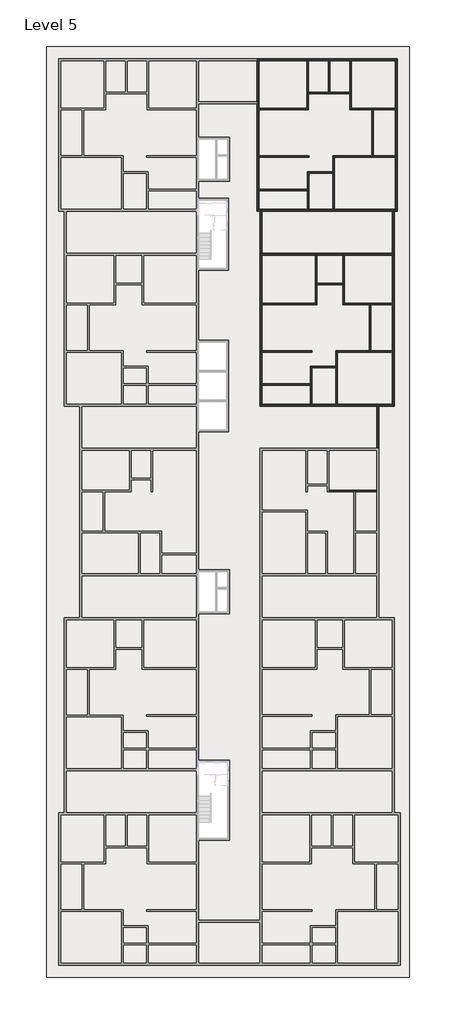
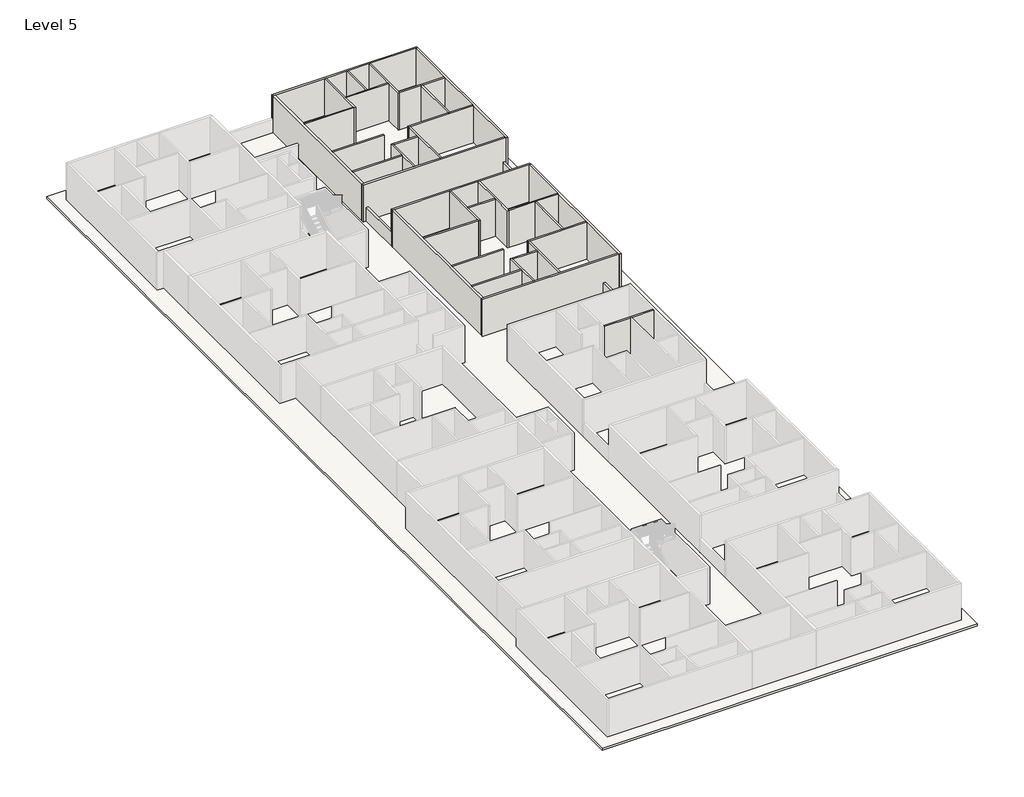
# One storey, part 4 of 8: 37 walls, 1 roof, 1 slab.
"""IFC4 building model written with IfcOpenShell, lengths in millimetres."""

from ifc_helpers import new_model, si_unit, frame, origin, place, context, project, spatial, polyline, outline, extrude, faceted_brep, element, save

model = new_model("IFC4")

# Units and contexts
model_context = context("Model", 3, world=origin())
ifc_project = project(units=[si_unit("LENGTHUNIT", "METRE", prefix="MILLI")], contexts=[model_context])

# Site, building, storey
site = spatial("IfcSite", under=ifc_project)
building = spatial("IfcBuilding", under=site)
storey = spatial("IfcBuildingStorey", under=building, Name="Level 5", Elevation=37426.6172466)

# Roof
placement = place(None, origin())
element("IfcRoof", 1, ObjectType="SLAB", at=placement, inside=storey, context=model_context, shape_type="SweptSolid", body=[
    extrude(outline(polyline([(-15237.9415084, -35021.5344126), (-15237.9415084, 36097.9216096), (12498.9443719, 36097.9216096), (12498.9443719, -35021.5344126), (-15237.9415084, -35021.5344126)]), holes=[polyline([(-3617.4415084, 29152.4900967), (-3617.4415084, 25799.6900967), (-1255.2415084, 25799.6900967), (-1255.2415084, 29152.4900967), (-3617.4415084, 29152.4900967)]), polyline([(-3617.4415084, 24490.1216096), (-3617.4415084, 19003.7216096), (-1331.4415084, 19003.7216096), (-1331.4415084, 24490.1216096), (-3617.4415084, 24490.1216096)]), polyline([(-3617.4415084, 13669.6303368), (-3617.4415084, 6659.2303368), (-1331.4415084, 6659.2303368), (-1331.4415084, 13669.6303368), (-3617.4415084, 13669.6303368)]), polyline([(-3617.4415084, -3882.2751812), (-3617.4415084, -7235.0751812), (-1255.2415084, -7235.0751812), (-1255.2415084, -3882.2751812), (-3617.4415084, -3882.2751812)]), polyline([(-3617.4415084, -18429.9851539), (-3617.4415084, -24525.9851539), (-1229.8415084, -24525.9851539), (-1229.8415084, -18429.9851539), (-3617.4415084, -18429.9851539)])]), frame((0.0, 0.0, 37426.6172466), z_axis=(0.0, 0.0, 1.0), x_axis=(1.0, 0.0, 0.0)), (0.0, 0.0, 1.0), 152.4),
])

# Slab
element("IfcSlab", 2, ObjectType="FLOOR", at=placement, inside=storey, context=model_context, shape_type="SweptSolid", body=[
    extrude(outline(polyline([(-14323.5415084, 35183.5216096), (11584.5443719, 35183.5216096), (11584.5443719, 23499.5216096), (11360.9214687, 23499.5216096), (11360.9214687, 8615.1216096), (10173.4714687, 8615.1216096), (10173.4714687, -7538.7344126), (11360.9214687, -7538.7344126), (11360.9214687, -22423.1344126), (11813.0584916, -22423.1344126), (11813.0584916, -34107.1344126), (11584.5443719, -34107.1344126), (-14323.5415084, -34107.1344126), (-14323.5415084, 35183.5216096)]), holes=[polyline([(-3617.4415084, 29152.4900967), (-3617.4415084, 25799.6900967), (-1255.2415084, 25799.6900967), (-1255.2415084, 29152.4900967), (-3617.4415084, 29152.4900967)]), polyline([(-3617.4415084, 24490.1216096), (-3617.4415084, 19003.7216096), (-1331.4415084, 19003.7216096), (-1331.4415084, 24490.1216096), (-3617.4415084, 24490.1216096)]), polyline([(-3617.4415084, 13669.6303368), (-3617.4415084, 6659.2303368), (-1331.4415084, 6659.2303368), (-1331.4415084, 13669.6303368), (-3617.4415084, 13669.6303368)]), polyline([(-3617.4415084, -3882.2751812), (-3617.4415084, -7235.0751812), (-1255.2415084, -7235.0751812), (-1255.2415084, -3882.2751812), (-3617.4415084, -3882.2751812)]), polyline([(-3617.4415084, -18429.9851539), (-3617.4415084, -24525.9851539), (-1229.8415084, -24525.9851539), (-1229.8415084, -18429.9851539), (-3617.4415084, -18429.9851539)])]), frame((0.0, 0.0, 36817.0172466), z_axis=(0.0, 0.0, 1.0), x_axis=(1.0, 0.0, 0.0)), (0.0, 0.0, 1.0), 609.6),
])

# Walls
element("IfcWall", 3, ObjectType="4.5\"", at=placement, inside=storey, context=model_context, shape_type="Brep", body=[
    faceted_brep([(6363.4714687, 2100.0216096, 37426.6172466), (8282.4584916, 2100.0216096, 37426.6172466), (8396.7584916, 2100.0216096, 37426.6172466), (10021.0714687, 2100.0216096, 37426.6172466), (10021.0714687, 2100.0216096, 40474.6172466), (8396.7584916, 2100.0216096, 40474.6172466), (8282.4584916, 2100.0216096, 40474.6172466), (6363.4714687, 2100.0216096, 40474.6172466), (6363.4714687, 2214.3216096, 37426.6172466), (6363.4714687, 2214.3216096, 40474.6172466), (10021.0714687, 2214.3216096, 40474.6172466), (10021.0714687, 2214.3216096, 37426.6172466)], [[[0, 1, 2, 3, 4, 5, 6, 7]], [[8, 9, 10, 11]], [[3, 2, 1, 0, 8, 11]], [[0, 7, 9, 8]], [[4, 3, 11, 10]], [[7, 6, 5, 4, 10, 9]]]),
])
element("IfcWall", 4, ObjectType="4.5\"", at=placement, inside=storey, context=model_context, shape_type="Brep", body=[
    faceted_brep([(5315.7214687, 20146.7216096, 37426.6172466), (5315.7214687, 16489.1216096, 37426.6172466), (5315.7214687, 16374.8216096, 37426.6172466), (5315.7214687, 16374.8216096, 40474.6172466), (5315.7214687, 16489.1216096, 40474.6172466), (5315.7214687, 20146.7216096, 40474.6172466), (5430.0214687, 20146.7216096, 37426.6172466), (5430.0214687, 20146.7216096, 40474.6172466), (5430.0214687, 18013.1216096, 40474.6172466), (5430.0214687, 17898.8216096, 40474.6172466), (5430.0214687, 16374.8216096, 40474.6172466), (5430.0214687, 16374.8216096, 37426.6172466), (5430.0214687, 17898.8216096, 37426.6172466), (5430.0214687, 18013.1216096, 37426.6172466)], [[[0, 1, 2, 3, 4, 5]], [[6, 7, 8, 9, 10, 11, 12, 13]], [[2, 1, 0, 6, 13, 12, 11]], [[0, 5, 7, 6]], [[3, 2, 11, 10]], [[5, 4, 3, 10, 9, 8, 7]]]),
])
element("IfcWall", 5, ObjectType="4.5\"", at=placement, inside=storey, context=model_context, shape_type="SweptSolid", body=[
    extrude(outline(polyline([(1259.3584916, 16489.1216096), (5315.7214687, 16489.1216096), (5315.7214687, 16374.8216096), (1259.3584916, 16374.8216096), (1259.3584916, 16489.1216096)])), frame((0.0, 0.0, 37426.6172466), z_axis=(0.0, 0.0, 1.0), x_axis=(1.0, 0.0, 0.0)), (0.0, 0.0, 1.0), 3048.0),
])
element("IfcWall", 6, ObjectType="4.5\"", at=placement, inside=storey, context=model_context, shape_type="SweptSolid", body=[
    extrude(outline(polyline([(7436.6214687, 17898.8216096), (5430.0214687, 17898.8216096), (5430.0214687, 18013.1216096), (7436.6214687, 18013.1216096), (7436.6214687, 17898.8216096)])), frame((0.0, 0.0, 37426.6172466), z_axis=(0.0, 0.0, 1.0), x_axis=(1.0, 0.0, 0.0)), (0.0, 0.0, 1.0), 3048.0),
])
element("IfcWall", 7, ObjectType="4.5\"", at=placement, inside=storey, context=model_context, shape_type="Brep", body=[
    faceted_brep([(7436.6214687, 20146.7216096, 37426.6172466), (7436.6214687, 18013.1216096, 37426.6172466), (7436.6214687, 17898.8216096, 37426.6172466), (7436.6214687, 16374.8216096, 37426.6172466), (7436.6214687, 16374.8216096, 40474.6172466), (7436.6214687, 17898.8216096, 40474.6172466), (7436.6214687, 18013.1216096, 40474.6172466), (7436.6214687, 20146.7216096, 40474.6172466), (7550.9214687, 20146.7216096, 37426.6172466), (7550.9214687, 20146.7216096, 40474.6172466), (7550.9214687, 16489.1216096, 40474.6172466), (7550.9214687, 16374.8216096, 40474.6172466), (7550.9214687, 16374.8216096, 37426.6172466), (7550.9214687, 16489.1216096, 37426.6172466)], [[[0, 1, 2, 3, 4, 5, 6, 7]], [[8, 9, 10, 11, 12, 13]], [[3, 2, 1, 0, 8, 13, 12]], [[0, 7, 9, 8]], [[4, 3, 12, 11]], [[7, 6, 5, 4, 11, 10, 9]]]),
])
element("IfcWall", 8, ObjectType="4.5\"", at=placement, inside=storey, context=model_context, shape_type="Brep", body=[
    faceted_brep([(7550.9214687, 16374.8216096, 37426.6172466), (9469.9084916, 16374.8216096, 37426.6172466), (9584.2084916, 16374.8216096, 37426.6172466), (11208.5214687, 16374.8216096, 37426.6172466), (11208.5214687, 16374.8216096, 40474.6172466), (9584.2084916, 16374.8216096, 40474.6172466), (9469.9084916, 16374.8216096, 40474.6172466), (7550.9214687, 16374.8216096, 40474.6172466), (7550.9214687, 16489.1216096, 37426.6172466), (7550.9214687, 16489.1216096, 40474.6172466), (11208.5214687, 16489.1216096, 40474.6172466), (11208.5214687, 16489.1216096, 37426.6172466)], [[[0, 1, 2, 3, 4, 5, 6, 7]], [[8, 9, 10, 11]], [[3, 2, 1, 0, 8, 11]], [[0, 7, 9, 8]], [[4, 3, 11, 10]], [[7, 6, 5, 4, 10, 9]]]),
])
element("IfcWall", 9, ObjectType="4.5\"", at=placement, inside=storey, context=model_context, shape_type="SweptSolid", body=[
    extrude(outline(polyline([(9469.9084916, 12869.6216096), (9469.9084916, 16374.8216096), (9584.2084916, 16374.8216096), (9584.2084916, 12869.6216096), (9469.9084916, 12869.6216096)])), frame((0.0, 0.0, 37426.6172466), z_axis=(0.0, 0.0, 1.0), x_axis=(1.0, 0.0, 0.0)), (0.0, 0.0, 1.0), 3048.0),
])
element("IfcWall", 10, ObjectType="4.5\"", at=placement, inside=storey, context=model_context, shape_type="Brep", body=[
    faceted_brep([(11208.5214687, 12869.6216096, 37426.6172466), (9584.2084916, 12869.6216096, 37426.6172466), (9469.9084916, 12869.6216096, 37426.6172466), (6885.4584916, 12869.6216096, 37426.6172466), (6885.4584916, 12869.6216096, 40474.6172466), (9469.9084916, 12869.6216096, 40474.6172466), (9584.2084916, 12869.6216096, 40474.6172466), (11208.5214687, 12869.6216096, 40474.6172466), (11208.5214687, 12755.3216096, 37426.6172466), (11208.5214687, 12755.3216096, 40474.6172466), (6999.7584916, 12755.3216096, 40474.6172466), (6885.4584916, 12755.3216096, 40474.6172466), (6885.4584916, 12755.3216096, 37426.6172466), (6999.7584916, 12755.3216096, 37426.6172466)], [[[0, 1, 2, 3, 4, 5, 6, 7]], [[8, 9, 10, 11, 12, 13]], [[3, 2, 1, 0, 8, 13, 12]], [[0, 7, 9, 8]], [[4, 3, 12, 11]], [[7, 6, 5, 4, 11, 10, 9]]]),
])
element("IfcWall", 11, ObjectType="4.5\"", at=placement, inside=storey, context=model_context, shape_type="Brep", body=[
    faceted_brep([(6885.4584916, 12755.3216096, 37426.6172466), (6885.4584916, 11663.1216096, 37426.6172466), (6885.4584916, 11548.8216096, 37426.6172466), (6885.4584916, 8767.5216096, 37426.6172466), (6885.4584916, 8767.5216096, 40474.6172466), (6885.4584916, 11548.8216096, 40474.6172466), (6885.4584916, 11663.1216096, 40474.6172466), (6885.4584916, 12755.3216096, 40474.6172466), (6999.7584916, 12755.3216096, 37426.6172466), (6999.7584916, 12755.3216096, 40474.6172466), (6999.7584916, 8767.5216096, 40474.6172466), (6999.7584916, 8767.5216096, 37426.6172466)], [[[0, 1, 2, 3, 4, 5, 6, 7]], [[8, 9, 10, 11]], [[3, 2, 1, 0, 8, 11]], [[0, 7, 9, 8]], [[4, 3, 11, 10]], [[7, 6, 5, 4, 10, 9]]]),
])
element("IfcWall", 12, ObjectType="4.5\"", at=placement, inside=storey, context=model_context, shape_type="Brep", body=[
    faceted_brep([(5056.6584916, 8767.5216096, 37426.6172466), (5056.6584916, 11548.8216096, 37426.6172466), (5056.6584916, 11663.1216096, 37426.6172466), (5056.6584916, 11663.1216096, 40474.6172466), (5056.6584916, 11548.8216096, 40474.6172466), (5056.6584916, 8767.5216096, 40474.6172466), (4942.3584916, 8767.5216096, 37426.6172466), (4942.3584916, 8767.5216096, 40474.6172466), (4942.3584916, 10215.3216096, 40474.6172466), (4942.3584916, 10329.6216096, 40474.6172466), (4942.3584916, 11663.1216096, 40474.6172466), (4942.3584916, 11663.1216096, 37426.6172466), (4942.3584916, 10329.6216096, 37426.6172466), (4942.3584916, 10215.3216096, 37426.6172466)], [[[0, 1, 2, 3, 4, 5]], [[6, 7, 8, 9, 10, 11, 12, 13]], [[2, 1, 0, 6, 13, 12, 11]], [[0, 5, 7, 6]], [[3, 2, 11, 10]], [[5, 4, 3, 10, 9, 8, 7]]]),
])
element("IfcWall", 13, ObjectType="4.5\"", at=placement, inside=storey, context=model_context, shape_type="SweptSolid", body=[
    extrude(outline(polyline([(6885.4584916, 11548.8216096), (5056.6584916, 11548.8216096), (5056.6584916, 11663.1216096), (6885.4584916, 11663.1216096), (6885.4584916, 11548.8216096)])), frame((0.0, 0.0, 37426.6172466), z_axis=(0.0, 0.0, 1.0), x_axis=(1.0, 0.0, 0.0)), (0.0, 0.0, 1.0), 3048.0),
])
element("IfcWall", 14, ObjectType="4.5\"", at=placement, inside=storey, context=model_context, shape_type="SweptSolid", body=[
    extrude(outline(polyline([(4942.3584916, 10215.3216096), (1259.3584916, 10215.3216096), (1259.3584916, 10329.6216096), (4942.3584916, 10329.6216096), (4942.3584916, 10215.3216096)])), frame((0.0, 0.0, 37426.6172466), z_axis=(0.0, 0.0, 1.0), x_axis=(1.0, 0.0, 0.0)), (0.0, 0.0, 1.0), 3048.0),
])
element("IfcWall", 15, ObjectType="4.5\"", at=placement, inside=storey, context=model_context, shape_type="SweptSolid", body=[
    extrude(outline(polyline([(5056.6584916, 12755.3216096), (1259.3584916, 12755.3216096), (1259.3584916, 12869.6216096), (5056.6584916, 12869.6216096), (5056.6584916, 12755.3216096)])), frame((0.0, 0.0, 37426.6172466), z_axis=(0.0, 0.0, 1.0), x_axis=(1.0, 0.0, 0.0)), (0.0, 0.0, 1.0), 3048.0),
])
element("IfcWall", 16, ObjectType="4.5\"", at=placement, inside=storey, context=model_context, shape_type="Brep", body=[
    faceted_brep([(4688.4443719, 35031.1216096, 37426.6172466), (4688.4443719, 31373.5216096, 37426.6172466), (4688.4443719, 31259.2216096, 37426.6172466), (4688.4443719, 31259.2216096, 40474.6172466), (4688.4443719, 31373.5216096, 40474.6172466), (4688.4443719, 35031.1216096, 40474.6172466), (4802.7443719, 35031.1216096, 37426.6172466), (4802.7443719, 35031.1216096, 40474.6172466), (4802.7443719, 32592.7216096, 40474.6172466), (4802.7443719, 32478.4216096, 40474.6172466), (4802.7443719, 31259.2216096, 40474.6172466), (4802.7443719, 31259.2216096, 37426.6172466), (4802.7443719, 32478.4216096, 37426.6172466), (4802.7443719, 32592.7216096, 37426.6172466)], [[[0, 1, 2, 3, 4, 5]], [[6, 7, 8, 9, 10, 11, 12, 13]], [[2, 1, 0, 6, 13, 12, 11]], [[0, 5, 7, 6]], [[3, 2, 11, 10]], [[5, 4, 3, 10, 9, 8, 7]]]),
])
element("IfcWall", 17, ObjectType="4.5\"", at=placement, inside=storey, context=model_context, shape_type="SweptSolid", body=[
    extrude(outline(polyline([(1030.8443719, 31373.5216096), (4688.4443719, 31373.5216096), (4688.4443719, 31259.2216096), (1030.8443719, 31259.2216096), (1030.8443719, 31373.5216096)])), frame((0.0, 0.0, 37426.6172466), z_axis=(0.0, 0.0, 1.0), x_axis=(1.0, 0.0, 0.0)), (0.0, 0.0, 1.0), 3048.0),
])
element("IfcWall", 18, ObjectType="4.5\"", at=placement, inside=storey, context=model_context, shape_type="Brep", body=[
    faceted_brep([(4802.7443719, 32478.4216096, 37426.6172466), (7965.0443719, 32478.4216096, 37426.6172466), (7965.0443719, 32478.4216096, 40474.6172466), (4802.7443719, 32478.4216096, 40474.6172466), (4802.7443719, 32592.7216096, 37426.6172466), (4802.7443719, 32592.7216096, 40474.6172466), (6326.7443719, 32592.7216096, 40474.6172466), (6441.0443719, 32592.7216096, 40474.6172466), (7965.0443719, 32592.7216096, 40474.6172466), (7965.0443719, 32592.7216096, 37426.6172466), (6441.0443719, 32592.7216096, 37426.6172466), (6326.7443719, 32592.7216096, 37426.6172466)], [[[0, 1, 2, 3]], [[4, 5, 6, 7, 8, 9, 10, 11]], [[1, 0, 4, 11, 10, 9]], [[0, 3, 5, 4]], [[2, 1, 9, 8]], [[3, 2, 8, 7, 6, 5]]]),
])
element("IfcWall", 19, ObjectType="4.5\"", at=placement, inside=storey, context=model_context, shape_type="SweptSolid", body=[
    extrude(outline(polyline([(6326.7443719, 32592.7216096), (6326.7443719, 35031.1216096), (6441.0443719, 35031.1216096), (6441.0443719, 32592.7216096), (6326.7443719, 32592.7216096)])), frame((0.0, 0.0, 37426.6172466), z_axis=(0.0, 0.0, 1.0), x_axis=(1.0, 0.0, 0.0)), (0.0, 0.0, 1.0), 3048.0),
])
element("IfcWall", 20, ObjectType="4.5\"", at=placement, inside=storey, context=model_context, shape_type="Brep", body=[
    faceted_brep([(7965.0443719, 35031.1216096, 37426.6172466), (7965.0443719, 32592.7216096, 37426.6172466), (7965.0443719, 32478.4216096, 37426.6172466), (7965.0443719, 31259.2216096, 37426.6172466), (7965.0443719, 31259.2216096, 40474.6172466), (7965.0443719, 32478.4216096, 40474.6172466), (7965.0443719, 32592.7216096, 40474.6172466), (7965.0443719, 35031.1216096, 40474.6172466), (8079.3443719, 35031.1216096, 37426.6172466), (8079.3443719, 35031.1216096, 40474.6172466), (8079.3443719, 31373.5216096, 40474.6172466), (8079.3443719, 31259.2216096, 40474.6172466), (8079.3443719, 31259.2216096, 37426.6172466), (8079.3443719, 31373.5216096, 37426.6172466)], [[[0, 1, 2, 3, 4, 5, 6, 7]], [[8, 9, 10, 11, 12, 13]], [[3, 2, 1, 0, 8, 13, 12]], [[0, 7, 9, 8]], [[4, 3, 12, 11]], [[7, 6, 5, 4, 11, 10, 9]]]),
])
element("IfcWall", 21, ObjectType="4.5\"", at=placement, inside=storey, context=model_context, shape_type="Brep", body=[
    faceted_brep([(8079.3443719, 31259.2216096, 37426.6172466), (9641.4443719, 31259.2216096, 37426.6172466), (9755.7443719, 31259.2216096, 37426.6172466), (11432.1443719, 31259.2216096, 37426.6172466), (11432.1443719, 31259.2216096, 40474.6172466), (9755.7443719, 31259.2216096, 40474.6172466), (9641.4443719, 31259.2216096, 40474.6172466), (8079.3443719, 31259.2216096, 40474.6172466), (8079.3443719, 31373.5216096, 37426.6172466), (8079.3443719, 31373.5216096, 40474.6172466), (11432.1443719, 31373.5216096, 40474.6172466), (11432.1443719, 31373.5216096, 37426.6172466)], [[[0, 1, 2, 3, 4, 5, 6, 7]], [[8, 9, 10, 11]], [[3, 2, 1, 0, 8, 11]], [[0, 7, 9, 8]], [[4, 3, 11, 10]], [[7, 6, 5, 4, 10, 9]]]),
])
element("IfcWall", 22, ObjectType="4.5\"", at=placement, inside=storey, context=model_context, shape_type="SweptSolid", body=[
    extrude(outline(polyline([(9641.4443719, 27754.0216096), (9641.4443719, 31259.2216096), (9755.7443719, 31259.2216096), (9755.7443719, 27754.0216096), (9641.4443719, 27754.0216096)])), frame((0.0, 0.0, 37426.6172466), z_axis=(0.0, 0.0, 1.0), x_axis=(1.0, 0.0, 0.0)), (0.0, 0.0, 1.0), 3048.0),
])
element("IfcWall", 23, ObjectType="4.5\"", at=placement, inside=storey, context=model_context, shape_type="Brep", body=[
    faceted_brep([(11432.1443719, 27754.0216096, 37426.6172466), (9755.7443719, 27754.0216096, 37426.6172466), (9641.4443719, 27754.0216096, 37426.6172466), (6656.9443719, 27754.0216096, 37426.6172466), (6656.9443719, 27754.0216096, 40474.6172466), (9641.4443719, 27754.0216096, 40474.6172466), (9755.7443719, 27754.0216096, 40474.6172466), (11432.1443719, 27754.0216096, 40474.6172466), (11432.1443719, 27639.7216096, 37426.6172466), (11432.1443719, 27639.7216096, 40474.6172466), (6771.2443719, 27639.7216096, 40474.6172466), (6656.9443719, 27639.7216096, 40474.6172466), (6656.9443719, 27639.7216096, 37426.6172466), (6771.2443719, 27639.7216096, 37426.6172466)], [[[0, 1, 2, 3, 4, 5, 6, 7]], [[8, 9, 10, 11, 12, 13]], [[3, 2, 1, 0, 8, 13, 12]], [[0, 7, 9, 8]], [[4, 3, 12, 11]], [[7, 6, 5, 4, 11, 10, 9]]]),
])
element("IfcWall", 24, ObjectType="4.5\"", at=placement, inside=storey, context=model_context, shape_type="Brep", body=[
    faceted_brep([(6656.9443719, 27639.7216096, 37426.6172466), (6656.9443719, 26547.5216096, 37426.6172466), (6656.9443719, 26433.2216096, 37426.6172466), (6656.9443719, 23651.9216096, 37426.6172466), (6656.9443719, 23651.9216096, 40474.6172466), (6656.9443719, 26433.2216096, 40474.6172466), (6656.9443719, 26547.5216096, 40474.6172466), (6656.9443719, 27639.7216096, 40474.6172466), (6771.2443719, 27639.7216096, 37426.6172466), (6771.2443719, 27639.7216096, 40474.6172466), (6771.2443719, 23651.9216096, 40474.6172466), (6771.2443719, 23651.9216096, 37426.6172466)], [[[0, 1, 2, 3, 4, 5, 6, 7]], [[8, 9, 10, 11]], [[3, 2, 1, 0, 8, 11]], [[0, 7, 9, 8]], [[4, 3, 11, 10]], [[7, 6, 5, 4, 10, 9]]]),
])
element("IfcWall", 25, ObjectType="4.5\"", at=placement, inside=storey, context=model_context, shape_type="SweptSolid", body=[
    extrude(outline(polyline([(4713.8443719, 25099.7216096), (1030.8443719, 25099.7216096), (1030.8443719, 25214.0216096), (4713.8443719, 25214.0216096), (4713.8443719, 25099.7216096)])), frame((0.0, 0.0, 37426.6172466), z_axis=(0.0, 0.0, 1.0), x_axis=(1.0, 0.0, 0.0)), (0.0, 0.0, 1.0), 3048.0),
])
element("IfcWall", 26, ObjectType="4.5\"", at=placement, inside=storey, context=model_context, shape_type="Brep", body=[
    faceted_brep([(4828.1443719, 23651.9216096, 37426.6172466), (4828.1443719, 26433.2216096, 37426.6172466), (4828.1443719, 26547.5216096, 37426.6172466), (4828.1443719, 26547.5216096, 40474.6172466), (4828.1443719, 26433.2216096, 40474.6172466), (4828.1443719, 23651.9216096, 40474.6172466), (4713.8443719, 23651.9216096, 37426.6172466), (4713.8443719, 23651.9216096, 40474.6172466), (4713.8443719, 25099.7216096, 40474.6172466), (4713.8443719, 25214.0216096, 40474.6172466), (4713.8443719, 26547.5216096, 40474.6172466), (4713.8443719, 26547.5216096, 37426.6172466), (4713.8443719, 25214.0216096, 37426.6172466), (4713.8443719, 25099.7216096, 37426.6172466)], [[[0, 1, 2, 3, 4, 5]], [[6, 7, 8, 9, 10, 11, 12, 13]], [[2, 1, 0, 6, 13, 12, 11]], [[0, 5, 7, 6]], [[3, 2, 11, 10]], [[5, 4, 3, 10, 9, 8, 7]]]),
])
element("IfcWall", 27, ObjectType="4.5\"", at=placement, inside=storey, context=model_context, shape_type="SweptSolid", body=[
    extrude(outline(polyline([(6656.9443719, 26433.2216096), (4828.1443719, 26433.2216096), (4828.1443719, 26547.5216096), (6656.9443719, 26547.5216096), (6656.9443719, 26433.2216096)])), frame((0.0, 0.0, 37426.6172466), z_axis=(0.0, 0.0, 1.0), x_axis=(1.0, 0.0, 0.0)), (0.0, 0.0, 1.0), 3048.0),
])
element("IfcWall", 28, ObjectType="4.5\"", at=placement, inside=storey, context=model_context, shape_type="SweptSolid", body=[
    extrude(outline(polyline([(4828.1443719, 27639.7216096), (1030.8443719, 27639.7216096), (1030.8443719, 27754.0216096), (4828.1443719, 27754.0216096), (4828.1443719, 27639.7216096)])), frame((0.0, 0.0, 37426.6172466), z_axis=(0.0, 0.0, 1.0), x_axis=(1.0, 0.0, 0.0)), (0.0, 0.0, 1.0), 3048.0),
])
element("IfcWall", 29, ObjectType="6\"", at=placement, inside=storey, context=model_context, shape_type="Brep", body=[
    faceted_brep([(1106.9584916, 20146.7216096, 40474.6172466), (1106.9584916, 20146.7216096, 37426.6172466), (1259.3584916, 20146.7216096, 37426.6172466), (5315.7214687, 20146.7216096, 37426.6172466), (5430.0214687, 20146.7216096, 37426.6172466), (7436.6214687, 20146.7216096, 37426.6172466), (7550.9214687, 20146.7216096, 37426.6172466), (11208.5214687, 20146.7216096, 37426.6172466), (11360.9214687, 20146.7216096, 37426.6172466), (11360.9214687, 20146.7216096, 40474.6172466), (11208.5214687, 20146.7216096, 40474.6172466), (7550.9214687, 20146.7216096, 40474.6172466), (7436.6214687, 20146.7216096, 40474.6172466), (5430.0214687, 20146.7216096, 40474.6172466), (5315.7214687, 20146.7216096, 40474.6172466), (1259.3584916, 20146.7216096, 40474.6172466), (1106.9584916, 20299.1216096, 37426.6172466), (1106.9584916, 20299.1216096, 38645.8172466), (1106.9584916, 20299.1216096, 40474.6172466), (11360.9214687, 20299.1216096, 40474.6172466), (11360.9214687, 20299.1216096, 38645.8172466), (11360.9214687, 20299.1216096, 37426.6172466), (11208.5214687, 20299.1216096, 37426.6172466), (1259.3584916, 20299.1216096, 37426.6172466)], [[[0, 1, 2, 3, 4, 5, 6, 7, 8, 9, 10, 11, 12, 13, 14, 15]], [[16, 17, 18, 19, 20, 21, 22, 23]], [[8, 7, 6, 5, 4, 3, 2, 1, 16, 23, 22, 21]], [[0, 18, 17, 16, 1]], [[8, 21, 20, 19, 9]], [[0, 15, 14, 13, 12, 11, 10, 9, 19, 18]]]),
])
element("IfcWall", 30, ObjectType="6\"", at=placement, inside=storey, context=model_context, shape_type="Brep", body=[
    faceted_brep([(11208.5214687, 20146.7216096, 40474.6172466), (11208.5214687, 20146.7216096, 37426.6172466), (11208.5214687, 16489.1216096, 37426.6172466), (11208.5214687, 16374.8216096, 37426.6172466), (11208.5214687, 12869.6216096, 37426.6172466), (11208.5214687, 12755.3216096, 37426.6172466), (11208.5214687, 8767.5216096, 37426.6172466), (11208.5214687, 8615.1216096, 37426.6172466), (11208.5214687, 8615.1216096, 40474.6172466), (11208.5214687, 8767.5216096, 40474.6172466), (11208.5214687, 12755.3216096, 40474.6172466), (11208.5214687, 12869.6216096, 40474.6172466), (11208.5214687, 16374.8216096, 40474.6172466), (11208.5214687, 16489.1216096, 40474.6172466), (11360.9214687, 20146.7216096, 37426.6172466), (11360.9214687, 20146.7216096, 40474.6172466), (11360.9214687, 8615.1216096, 40474.6172466), (11360.9214687, 8615.1216096, 37426.6172466)], [[[0, 1, 2, 3, 4, 5, 6, 7, 8, 9, 10, 11, 12, 13]], [[14, 15, 16, 17]], [[7, 6, 5, 4, 3, 2, 1, 14, 17]], [[8, 7, 17, 16]], [[0, 15, 14, 1]], [[0, 13, 12, 11, 10, 9, 8, 16, 15]]]),
])
element("IfcWall", 31, ObjectType="6\"", at=placement, inside=storey, context=model_context, shape_type="Brep", body=[
    faceted_brep([(11208.5214687, 8767.5216096, 37426.6172466), (6999.7584916, 8767.5216096, 37426.6172466), (6885.4584916, 8767.5216096, 37426.6172466), (5056.6584916, 8767.5216096, 37426.6172466), (4942.3584916, 8767.5216096, 37426.6172466), (1259.3584916, 8767.5216096, 37426.6172466), (1106.9584916, 8767.5216096, 37426.6172466), (1106.9584916, 8767.5216096, 40474.6172466), (1259.3584916, 8767.5216096, 40474.6172466), (4942.3584916, 8767.5216096, 40474.6172466), (5056.6584916, 8767.5216096, 40474.6172466), (6885.4584916, 8767.5216096, 40474.6172466), (6999.7584916, 8767.5216096, 40474.6172466), (11208.5214687, 8767.5216096, 40474.6172466), (11208.5214687, 8615.1216096, 37426.6172466), (11208.5214687, 8615.1216096, 40474.6172466), (1106.9584916, 8615.1216096, 40474.6172466), (1106.9584916, 8615.1216096, 37426.6172466), (10021.0714687, 8615.1216096, 37426.6172466), (10173.4714687, 8615.1216096, 37426.6172466)], [[[0, 1, 2, 3, 4, 5, 6, 7, 8, 9, 10, 11, 12, 13]], [[14, 15, 16, 17, 18, 19]], [[6, 5, 4, 3, 2, 1, 0, 14, 19, 18, 17]], [[0, 13, 15, 14]], [[7, 6, 17, 16]], [[13, 12, 11, 10, 9, 8, 7, 16, 15]]]),
])
element("IfcWall", 32, ObjectType="6\"", at=placement, inside=storey, context=model_context, shape_type="Brep", body=[
    faceted_brep([(1259.3584916, 8767.5216096, 37426.6172466), (1259.3584916, 10215.3216096, 37426.6172466), (1259.3584916, 10329.6216096, 37426.6172466), (1259.3584916, 12755.3216096, 37426.6172466), (1259.3584916, 12869.6216096, 37426.6172466), (1259.3584916, 16374.8216096, 37426.6172466), (1259.3584916, 16489.1216096, 37426.6172466), (1259.3584916, 20146.7216096, 37426.6172466), (1259.3584916, 20146.7216096, 40474.6172466), (1259.3584916, 16489.1216096, 40474.6172466), (1259.3584916, 16374.8216096, 40474.6172466), (1259.3584916, 12869.6216096, 40474.6172466), (1259.3584916, 12755.3216096, 40474.6172466), (1259.3584916, 10329.6216096, 40474.6172466), (1259.3584916, 10215.3216096, 40474.6172466), (1259.3584916, 8767.5216096, 40474.6172466), (1106.9584916, 8767.5216096, 37426.6172466), (1106.9584916, 8767.5216096, 40474.6172466), (1106.9584916, 20146.7216096, 40474.6172466), (1106.9584916, 20146.7216096, 37426.6172466)], [[[0, 1, 2, 3, 4, 5, 6, 7, 8, 9, 10, 11, 12, 13, 14, 15]], [[16, 17, 18, 19]], [[7, 6, 5, 4, 3, 2, 1, 0, 16, 19]], [[0, 15, 17, 16]], [[7, 19, 18, 8]], [[15, 14, 13, 12, 11, 10, 9, 8, 18, 17]]]),
])
element("IfcWall", 33, ObjectType="6\"", at=placement, inside=storey, context=model_context, shape_type="Brep", body=[
    faceted_brep([(878.4443719, 35031.1216096, 40474.6172466), (878.4443719, 35031.1216096, 37426.6172466), (1030.8443719, 35031.1216096, 37426.6172466), (4688.4443719, 35031.1216096, 37426.6172466), (4802.7443719, 35031.1216096, 37426.6172466), (6326.7443719, 35031.1216096, 37426.6172466), (6441.0443719, 35031.1216096, 37426.6172466), (7965.0443719, 35031.1216096, 37426.6172466), (8079.3443719, 35031.1216096, 37426.6172466), (11432.1443719, 35031.1216096, 37426.6172466), (11584.5443719, 35031.1216096, 37426.6172466), (11584.5443719, 35031.1216096, 40474.6172466), (11432.1443719, 35031.1216096, 40474.6172466), (8079.3443719, 35031.1216096, 40474.6172466), (7965.0443719, 35031.1216096, 40474.6172466), (6441.0443719, 35031.1216096, 40474.6172466), (6326.7443719, 35031.1216096, 40474.6172466), (4802.7443719, 35031.1216096, 40474.6172466), (4688.4443719, 35031.1216096, 40474.6172466), (1030.8443719, 35031.1216096, 40474.6172466), (878.4443719, 35183.5216096, 37426.6172466), (878.4443719, 35183.5216096, 40474.6172466), (11584.5443719, 35183.5216096, 40474.6172466), (11584.5443719, 35183.5216096, 37426.6172466)], [[[0, 1, 2, 3, 4, 5, 6, 7, 8, 9, 10, 11, 12, 13, 14, 15, 16, 17, 18, 19]], [[20, 21, 22, 23]], [[10, 9, 8, 7, 6, 5, 4, 3, 2, 1, 20, 23]], [[11, 10, 23, 22]], [[0, 21, 20, 1]], [[0, 19, 18, 17, 16, 15, 14, 13, 12, 11, 22, 21]]]),
])
element("IfcWall", 34, ObjectType="6\"", at=placement, inside=storey, context=model_context, shape_type="Brep", body=[
    faceted_brep([(11432.1443719, 35031.1216096, 37426.6172466), (11432.1443719, 31373.5216096, 37426.6172466), (11432.1443719, 31259.2216096, 37426.6172466), (11432.1443719, 27754.0216096, 37426.6172466), (11432.1443719, 27639.7216096, 37426.6172466), (11432.1443719, 23651.9216096, 37426.6172466), (11432.1443719, 23499.5216096, 37426.6172466), (11432.1443719, 23499.5216096, 40474.6172466), (11432.1443719, 23651.9216096, 40474.6172466), (11432.1443719, 27639.7216096, 40474.6172466), (11432.1443719, 27754.0216096, 40474.6172466), (11432.1443719, 31259.2216096, 40474.6172466), (11432.1443719, 31373.5216096, 40474.6172466), (11432.1443719, 35031.1216096, 40474.6172466), (11584.5443719, 35031.1216096, 37426.6172466), (11584.5443719, 35031.1216096, 40474.6172466), (11584.5443719, 23499.5216096, 40474.6172466), (11584.5443719, 23499.5216096, 37426.6172466)], [[[0, 1, 2, 3, 4, 5, 6, 7, 8, 9, 10, 11, 12, 13]], [[14, 15, 16, 17]], [[6, 5, 4, 3, 2, 1, 0, 14, 17]], [[0, 13, 15, 14]], [[7, 6, 17, 16]], [[13, 12, 11, 10, 9, 8, 7, 16, 15]]]),
])
element("IfcWall", 35, ObjectType="6\"", at=placement, inside=storey, context=model_context, shape_type="Brep", body=[
    faceted_brep([(11432.1443719, 23651.9216096, 37426.6172466), (6771.2443719, 23651.9216096, 37426.6172466), (6656.9443719, 23651.9216096, 37426.6172466), (4828.1443719, 23651.9216096, 37426.6172466), (4713.8443719, 23651.9216096, 37426.6172466), (1030.8443719, 23651.9216096, 37426.6172466), (878.4443719, 23651.9216096, 37426.6172466), (878.4443719, 23651.9216096, 40474.6172466), (1030.8443719, 23651.9216096, 40474.6172466), (4713.8443719, 23651.9216096, 40474.6172466), (4828.1443719, 23651.9216096, 40474.6172466), (6656.9443719, 23651.9216096, 40474.6172466), (6771.2443719, 23651.9216096, 40474.6172466), (11432.1443719, 23651.9216096, 40474.6172466), (11432.1443719, 23499.5216096, 37426.6172466), (11432.1443719, 23499.5216096, 40474.6172466), (878.4443719, 23499.5216096, 40474.6172466), (878.4443719, 23499.5216096, 37426.6172466), (1106.9584916, 23499.5216096, 37426.6172466), (1259.3584916, 23499.5216096, 37426.6172466), (11208.5214687, 23499.5216096, 37426.6172466), (11360.9214687, 23499.5216096, 37426.6172466)], [[[0, 1, 2, 3, 4, 5, 6, 7, 8, 9, 10, 11, 12, 13]], [[14, 15, 16, 17, 18, 19, 20, 21]], [[6, 5, 4, 3, 2, 1, 0, 14, 21, 20, 19, 18, 17]], [[0, 13, 15, 14]], [[7, 6, 17, 16]], [[13, 12, 11, 10, 9, 8, 7, 16, 15]]]),
])
element("IfcWall", 36, ObjectType="6\"", at=placement, inside=storey, context=model_context, shape_type="Brep", body=[
    faceted_brep([(1030.8443719, 23651.9216096, 37426.6172466), (1030.8443719, 25099.7216096, 37426.6172466), (1030.8443719, 25214.0216096, 37426.6172466), (1030.8443719, 27639.7216096, 37426.6172466), (1030.8443719, 27754.0216096, 37426.6172466), (1030.8443719, 31259.2216096, 37426.6172466), (1030.8443719, 31373.5216096, 37426.6172466), (1030.8443719, 35031.1216096, 37426.6172466), (1030.8443719, 35031.1216096, 40474.6172466), (1030.8443719, 31373.5216096, 40474.6172466), (1030.8443719, 31259.2216096, 40474.6172466), (1030.8443719, 27754.0216096, 40474.6172466), (1030.8443719, 27639.7216096, 40474.6172466), (1030.8443719, 25214.0216096, 40474.6172466), (1030.8443719, 25099.7216096, 40474.6172466), (1030.8443719, 23651.9216096, 40474.6172466), (878.4443719, 23651.9216096, 37426.6172466), (878.4443719, 23651.9216096, 40474.6172466), (878.4443719, 35031.1216096, 40474.6172466), (878.4443719, 35031.1216096, 37426.6172466), (878.4443719, 31897.3197155, 37426.6172466), (878.4443719, 31744.9197155, 37426.6172466)], [[[0, 1, 2, 3, 4, 5, 6, 7, 8, 9, 10, 11, 12, 13, 14, 15]], [[16, 17, 18, 19, 20, 21]], [[7, 6, 5, 4, 3, 2, 1, 0, 16, 21, 20, 19]], [[0, 15, 17, 16]], [[7, 19, 18, 8]], [[15, 14, 13, 12, 11, 10, 9, 8, 18, 17]]]),
])
element("IfcWall", 37, ObjectType="6\" 2", at=placement, inside=storey, context=model_context, shape_type="SweptSolid", body=[
    extrude(outline(polyline([(1106.9584916, 20299.1216096), (1106.9584916, 23499.5216096), (1259.3584916, 23499.5216096), (1259.3584916, 20299.1216096), (1106.9584916, 20299.1216096)])), frame((0.0, 0.0, 37426.6172466), z_axis=(0.0, 0.0, 1.0), x_axis=(1.0, 0.0, 0.0)), (0.0, 0.0, 1.0), 1219.2),
])
element("IfcWall", 38, ObjectType="6\" 2", at=placement, inside=storey, context=model_context, shape_type="SweptSolid", body=[
    extrude(outline(polyline([(11208.5214687, 20299.1216096), (11208.5214687, 23499.5216096), (11360.9214687, 23499.5216096), (11360.9214687, 20299.1216096), (11208.5214687, 20299.1216096)])), frame((0.0, 0.0, 37426.6172466), z_axis=(0.0, 0.0, 1.0), x_axis=(1.0, 0.0, 0.0)), (0.0, 0.0, 1.0), 1219.2),
])
element("IfcWall", 39, ObjectType="6\" 2", at=placement, inside=storey, context=model_context, shape_type="SweptSolid", body=[
    extrude(outline(polyline([(10021.0714687, 5414.7216096), (10021.0714687, 8615.1216096), (10173.4714687, 8615.1216096), (10173.4714687, 5414.7216096), (10021.0714687, 5414.7216096)])), frame((0.0, 0.0, 37426.6172466), z_axis=(0.0, 0.0, 1.0), x_axis=(1.0, 0.0, 0.0)), (0.0, 0.0, 1.0), 1219.2),
])

save(model, "model.ifc")

# Revit data of these elements
# Type "SLAB"
#   Assembly Code = "B1020"
#   Layers, outside or top first: 0' - 6" "Damp-proofing" (function 1)
# Type "FLOOR"
#   Assembly Code = "B1010"
#   Function = 0
#   Layers, outside or top first: 2' - 0" "Tile, Porcelain, 4in" (function 1)
# Type "4.5\""
#   Assembly Code = "B2010"
#   Layers, outside or top first: 0' - 4 1/2" "WALLS" (function 1)
# Type "6\""
#   Assembly Code = "B2010"
#   Layers, outside or top first: 0' - 6" "WALLS" (function 1)
# Type "6\" 2"
#   Assembly Code = "B2010"
#   Layers, outside or top first: 0' - 6" "4'" (function 1)
# Element 1 (IfcRoof, "SLAB")
#   built-in parameter 1001705 = 123.291 (stored number, unit not read)
#   built-in parameter 1001710 = 33615
#   Phase Created = New Construction
#   Materials on its faces: "Damp-proofing"
# Element 2 (IfcSlab, "FLOOR")
#   built-in parameter 1001955 = 3.14159 (stored number, unit not read)
#   Height Offset From Level = 0' - 0"
#   Phase Created = New Construction
#   Materials on its faces: "Tile, Porcelain, 4in"
# Elements 3, 4, 5, 6, 7, 8, 9, 10, 11, 12, 13, 14, 15, 16, 17, 18, 19, 20, 21, 22, 23, 24, 25, 26, 27, 28 (IfcWall, "4.5\"")
#   Top Offset = 0' - 0"
#   Base Offset = 0' - 0"
#   Unconnected Height = 10' - 0"
#   wall height = 10' - 0"
#   Phase Created = New Construction
#   Base Constraint = Level 5
#   Materials on its faces: "WALLS"
# Elements 29, 30, 31, 32, 33, 34, 35, 36 (IfcWall, "6\"")
#   Top Offset = 0' - 0"
#   Base Offset = 0' - 0"
#   Unconnected Height = 10' - 0"
#   wall height = 10' - 0"
#   Phase Created = New Construction
#   Base Constraint = Level 5
#   Materials on its faces: "WALLS"
# Elements 37, 38, 39 (IfcWall, "6\" 2")
#   Top Offset = 0' - 0"
#   Base Offset = 0' - 0"
#   Unconnected Height = 4' - 0"
#   wall height = 4' - 0"
#   Phase Created = New Construction
#   Base Constraint = Level 5
#   Materials on its faces: "4'"
# Materials
#   "Damp-proofing": class "Generic", colour RGB 127 127 127, transparency 0, Description = "Damp-proofing", Cost = 0
#   "Tile, Porcelain, 4in": class "Generic", colour RGB 89 87 158, transparency 0, Description = "Porcelain tile, 4\", white", Cost = 0
#   "WALLS": class "Generic", colour RGB 120 120 120, transparency 0, Cost = 0
#   "4'": class "Generic", colour RGB 120 120 120, transparency 0, Cost = 0
